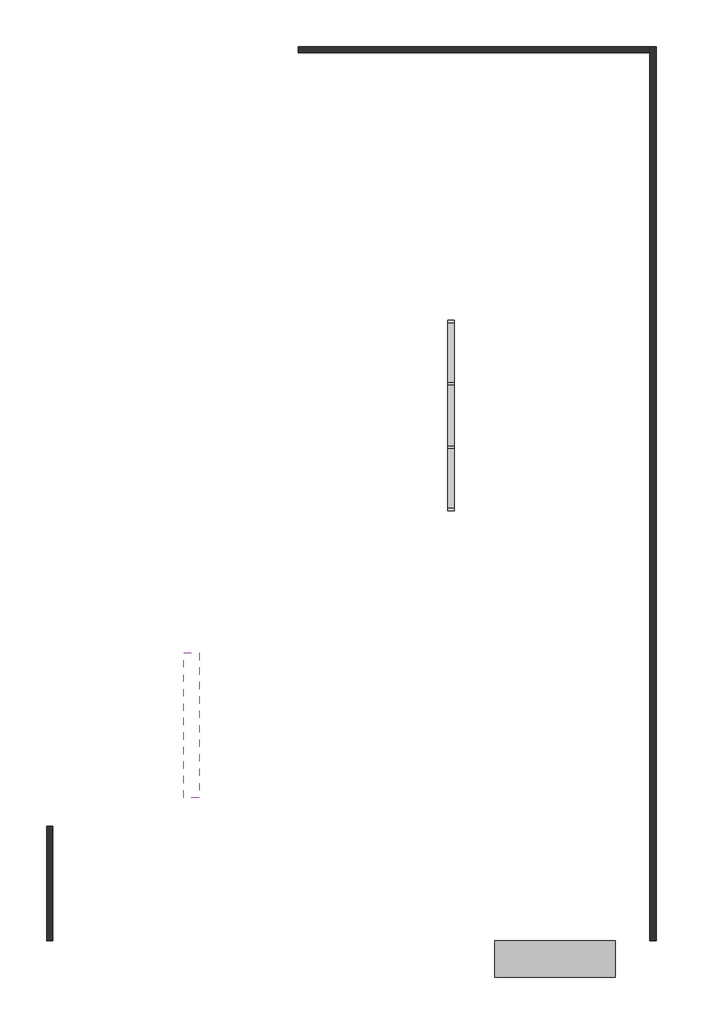
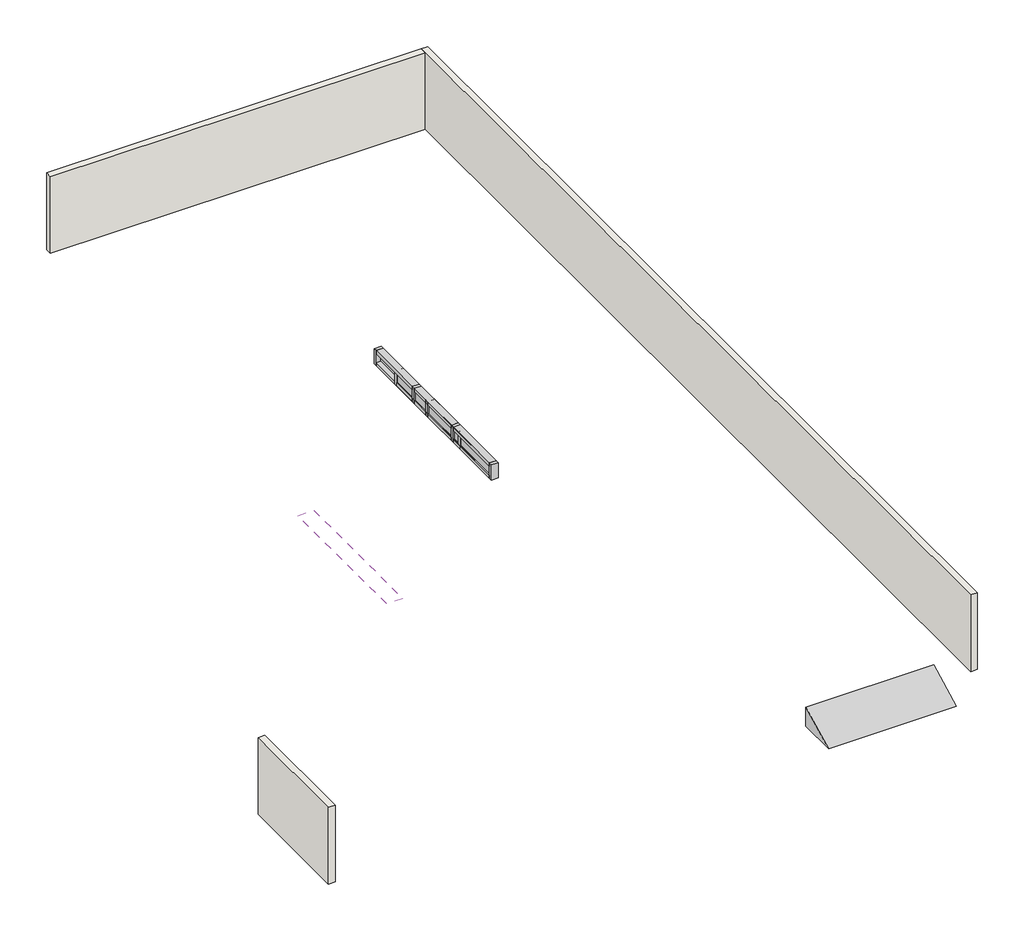
# One storey: 20 members, 6 plates, 3 walls, 1 covering, 1 proxy.
"""IFC4 building model written with IfcOpenShell, lengths in millimetres."""

from ifc_helpers import new_model, si_unit, frame, origin, place, context, project, spatial, polyline, outline, extrude, faceted_brep, transform, mapped, element, save
from components import generic_models_10_generic_models_10_e617d169, member_5d96a33e, member_91edd790, member_75d1e245, member_3c3dc66a, member_3b6b664d, member_f2556e69, system_panel_glazed_cafbbc3c, system_panel_glazed_d1fc495d, system_panel_glazed_eb071a3d, system_panel_glazed_471f9198

model = new_model("IFC4")

# Units and contexts
model_context = context("Model", 3, world=origin())
ifc_project = project(units=[si_unit("LENGTHUNIT", "METRE", prefix="MILLI")], contexts=[model_context])

# Site, building, storey
site = spatial("IfcSite", under=ifc_project)
building = spatial("IfcBuilding", under=site)
storey = spatial("IfcBuildingStorey", under=building, Elevation=0.0)

# Proxy
placement = place(None, origin())
generic_models_10_generic_models_10_shape = generic_models_10_generic_models_10_e617d169(model_context)
element("IfcBuildingElementProxy", 1, Name="Generic Models 10 : Generic Models 10", ObjectType="Generic Models 10 : Generic Models 10", at=placement, inside=storey, context=model_context, shape_type="MappedRepresentation", body=[
    mapped(generic_models_10_generic_models_10_shape, transform((0.0, 0.0, 0.0), x_axis=(1.0, 0.0, 0.0), y_axis=(0.0, 1.0, 0.0), z_axis=(0.0, 0.0, 1.0))),
])

# Covering
element("IfcCovering", 2, at=placement, inside=storey, context=model_context, shape_type="SweptSolid", body=[
    extrude(outline(polyline([(-4259.325552, -303.3614843), (-4259.325552, -3198.9614843), (-4564.125552, -3198.9614843), (-4564.125552, -303.3614843), (-4259.325552, -303.3614843)])), frame((0.0, 0.0, 2870.2), z_axis=(0.0, 0.0, 1.0), x_axis=(1.0, 0.0, 0.0)), (0.0, 0.0, 1.0), 41.275),
    extrude(outline(polyline([(-3649.725552, -303.3614843), (-3649.725552, -3198.9614843), (-3954.525552, -3198.9614843), (-3954.525552, -303.3614843), (-3649.725552, -303.3614843)])), frame((0.0, 0.0, 2870.2), z_axis=(0.0, 0.0, 1.0), x_axis=(1.0, 0.0, 0.0)), (0.0, 0.0, 1.0), 41.275),
    extrude(outline(polyline([(-3065.525552, -303.3614843), (-3065.525552, -3198.9614843), (-3370.325552, -3198.9614843), (-3370.325552, -303.3614843), (-3065.525552, -303.3614843)])), frame((0.0, 0.0, 2870.2), z_axis=(0.0, 0.0, 1.0), x_axis=(1.0, 0.0, 0.0)), (0.0, 0.0, 1.0), 41.275),
    extrude(outline(polyline([(-2455.925552, -303.3614843), (-2455.925552, -3198.9614843), (-2760.725552, -3198.9614843), (-2760.725552, -303.3614843), (-2455.925552, -303.3614843)])), frame((0.0, 0.0, 2870.2), z_axis=(0.0, 0.0, 1.0), x_axis=(1.0, 0.0, 0.0)), (0.0, 0.0, 1.0), 41.275),
    extrude(outline(polyline([(-1846.325552, -303.3614843), (-1846.325552, -3198.9614843), (-2151.125552, -3198.9614843), (-2151.125552, -303.3614843), (-1846.325552, -303.3614843)])), frame((0.0, 0.0, 2870.2), z_axis=(0.0, 0.0, 1.0), x_axis=(1.0, 0.0, 0.0)), (0.0, 0.0, 1.0), 41.275),
    extrude(outline(polyline([(-1236.725552, -303.3614843), (-1236.725552, -3198.9614843), (-1541.525552, -3198.9614843), (-1541.525552, -303.3614843), (-1236.725552, -303.3614843)])), frame((0.0, 0.0, 2870.2), z_axis=(0.0, 0.0, 1.0), x_axis=(1.0, 0.0, 0.0)), (0.0, 0.0, 1.0), 41.275),
])

# Members
member_shape = member_5d96a33e(model_context)
element("IfcMember", 3, ObjectType="Rectangular Mullion : 2.5\" x 5\" rectangular", at=placement, inside=storey, context=model_context, shape_type="MappedRepresentation", body=[
    mapped(member_shape, transform((781.026752, 2602.9133697, 304.8), x_axis=(0.0, 0.0, 1.0), y_axis=(-1.0, 0.0, 0.0), z_axis=(0.0, -1.0, 0.0))),
])
element("IfcMember", 4, ObjectType="Rectangular Mullion : 2.5\" x 5\" rectangular", at=placement, inside=storey, context=model_context, shape_type="MappedRepresentation", body=[
    mapped(member_shape, transform((781.026752, 5111.1633696, 304.8), x_axis=(0.0, 0.0, 1.0), y_axis=(-1.0, 0.0, 0.0), z_axis=(0.0, -1.0, 0.0))),
])
member_2_shape = member_91edd790(model_context)
element("IfcMember", 5, ObjectType="Rectangular Mullion : 2.5\" x 5\" rectangular", at=placement, inside=storey, context=model_context, shape_type="MappedRepresentation", body=[
    mapped(member_2_shape, transform((781.026752, 3841.1633698, 304.8), x_axis=(0.0, 0.0, 1.0), y_axis=(-1.0, 0.0, 0.0), z_axis=(0.0, -1.0, 0.0))),
])
element("IfcMember", 6, ObjectType="Rectangular Mullion : 2.5\" x 5\" rectangular", at=placement, inside=storey, context=model_context, shape_type="MappedRepresentation", body=[
    mapped(member_shape, transform((781.026752, 6285.9133697, 0.0), x_axis=(0.0, 0.0, -1.0), y_axis=(-1.0, 0.0, 0.0), z_axis=(0.0, 1.0, 0.0))),
])
element("IfcMember", 7, ObjectType="Rectangular Mullion : 2.5\" x 5\" rectangular", at=placement, inside=storey, context=model_context, shape_type="MappedRepresentation", body=[
    mapped(member_shape, transform((781.026752, 3777.6633698, 0.0), x_axis=(0.0, 0.0, -1.0), y_axis=(-1.0, 0.0, 0.0), z_axis=(0.0, 1.0, 0.0))),
])
element("IfcMember", 8, ObjectType="Rectangular Mullion : 2.5\" x 5\" rectangular", at=placement, inside=storey, context=model_context, shape_type="MappedRepresentation", body=[
    mapped(member_2_shape, transform((781.026752, 5047.6633696, 0.0), x_axis=(0.0, 0.0, -1.0), y_axis=(-1.0, 0.0, 0.0), z_axis=(0.0, 1.0, 0.0))),
])
member_3_shape = member_75d1e245(model_context)
element("IfcMember", 9, ObjectType="Rectangular Mullion : 2.5\" x 5\" rectangular", at=placement, inside=storey, context=model_context, shape_type="MappedRepresentation", body=[
    mapped(member_3_shape, transform((781.026752, 5079.4133696, 0.0), x_axis=(0.0, -1.0, 0.0), y_axis=(-1.0, 0.0, 0.0), z_axis=(0.0, 0.0, -1.0))),
])
element("IfcMember", 10, ObjectType="Rectangular Mullion : 2.5\" x 5\" rectangular", at=placement, inside=storey, context=model_context, shape_type="MappedRepresentation", body=[
    mapped(member_3_shape, transform((781.026752, 3809.4133698, 0.0), x_axis=(0.0, -1.0, 0.0), y_axis=(-1.0, 0.0, 0.0), z_axis=(0.0, 0.0, -1.0))),
])
element("IfcMember", 11, ObjectType="Rectangular Mullion : 2.5\" x 5\" rectangular", at=placement, inside=storey, context=model_context, shape_type="MappedRepresentation", body=[
    mapped(member_3_shape, transform((781.026752, 3589.2800365, 0.0), x_axis=(0.0, 1.0, 0.0), y_axis=(1.0, 0.0, 0.0), z_axis=(0.0, 0.0, -1.0))),
])
element("IfcMember", 12, ObjectType="Rectangular Mullion : 2.5\" x 5\" rectangular", at=placement, inside=storey, context=model_context, shape_type="MappedRepresentation", body=[
    mapped(member_3_shape, transform((781.026752, 4639.146703, 0.0), x_axis=(0.0, 1.0, 0.0), y_axis=(1.0, 0.0, 0.0), z_axis=(0.0, 0.0, -1.0))),
])
member_4_shape = member_3c3dc66a(model_context)
element("IfcMember", 13, ObjectType="Rectangular Mullion : 2.5\" x 5\" rectangular", at=placement, inside=storey, context=model_context, shape_type="MappedRepresentation", body=[
    mapped(member_4_shape, transform((781.026752, 2539.4133697, 0.0), x_axis=(0.0, -1.0, 0.0), y_axis=(-1.0, 0.0, 0.0), z_axis=(0.0, 0.0, -1.0))),
])
element("IfcMember", 14, ObjectType="Rectangular Mullion : 2.5\" x 5\" rectangular", at=placement, inside=storey, context=model_context, shape_type="MappedRepresentation", body=[
    mapped(member_4_shape, transform((781.026752, 5689.0133697, 0.0), x_axis=(0.0, 1.0, 0.0), y_axis=(1.0, 0.0, 0.0), z_axis=(0.0, 0.0, -1.0))),
])
element("IfcMember", 15, ObjectType="Rectangular Mullion : 2.5\" x 5\" rectangular", at=placement, inside=storey, context=model_context, shape_type="MappedRepresentation", body=[
    mapped(member_4_shape, transform((781.026752, 6349.4133697, 304.8), x_axis=(0.0, 1.0, 0.0), y_axis=(-1.0, 0.0, 0.0), z_axis=(0.0, 0.0, 1.0))),
])
element("IfcMember", 16, ObjectType="Rectangular Mullion : 2.5\" x 5\" rectangular", at=placement, inside=storey, context=model_context, shape_type="MappedRepresentation", body=[
    mapped(member_4_shape, transform((781.026752, 2539.4133697, 304.8), x_axis=(0.0, -1.0, 0.0), y_axis=(1.0, 0.0, 0.0), z_axis=(0.0, 0.0, 1.0))),
])
member_5_shape = member_3b6b664d(model_context)
element("IfcMember", 17, ObjectType="Rectangular Mullion : 2.5\" x 5\" rectangular", at=placement, inside=storey, context=model_context, shape_type="MappedRepresentation", body=[
    mapped(member_5_shape, transform((781.026752, 5625.5133697, 304.8), x_axis=(0.0, 0.0, 1.0), y_axis=(1.0, 0.0, 0.0), z_axis=(0.0, 1.0, 0.0))),
])
element("IfcMember", 18, ObjectType="Rectangular Mullion : 2.5\" x 5\" rectangular", at=placement, inside=storey, context=model_context, shape_type="MappedRepresentation", body=[
    mapped(member_5_shape, transform((781.026752, 3557.5300365, 304.8), x_axis=(0.0, 0.0, 1.0), y_axis=(1.0, 0.0, 0.0), z_axis=(0.0, 1.0, 0.0))),
])
member_6_shape = member_f2556e69(model_context)
element("IfcMember", 19, ObjectType="Rectangular Mullion : 2.5\" x 5\" rectangular", at=placement, inside=storey, context=model_context, shape_type="MappedRepresentation", body=[
    mapped(member_6_shape, transform((781.026752, 4607.396703, 304.8), x_axis=(0.0, 0.0, 1.0), y_axis=(1.0, 0.0, 0.0), z_axis=(0.0, 1.0, 0.0))),
])
element("IfcMember", 20, ObjectType="Rectangular Mullion : 2.5\" x 5\" rectangular", at=placement, inside=storey, context=model_context, shape_type="MappedRepresentation", body=[
    mapped(member_5_shape, transform((781.026752, 2602.9133697, 0.0), x_axis=(0.0, 0.0, -1.0), y_axis=(1.0, 0.0, 0.0), z_axis=(0.0, -1.0, 0.0))),
])
element("IfcMember", 21, ObjectType="Rectangular Mullion : 2.5\" x 5\" rectangular", at=placement, inside=storey, context=model_context, shape_type="MappedRepresentation", body=[
    mapped(member_5_shape, transform((781.026752, 4670.896703, 0.0), x_axis=(0.0, 0.0, -1.0), y_axis=(1.0, 0.0, 0.0), z_axis=(0.0, -1.0, 0.0))),
])
element("IfcMember", 22, ObjectType="Rectangular Mullion : 2.5\" x 5\" rectangular", at=placement, inside=storey, context=model_context, shape_type="MappedRepresentation", body=[
    mapped(member_6_shape, transform((781.026752, 3621.0300365, 0.0), x_axis=(0.0, 0.0, -1.0), y_axis=(1.0, 0.0, 0.0), z_axis=(0.0, -1.0, 0.0))),
])

# Plates
system_panel_glazed_shape = system_panel_glazed_cafbbc3c(model_context)
element("IfcPlate", 23, ObjectType="System Panel : Glazed", at=placement, inside=storey, context=model_context, shape_type="MappedRepresentation", body=[
    mapped(system_panel_glazed_shape, transform((781.026752, 5698.5383697, 63.5), x_axis=(0.0, -1.0, 0.0), y_axis=(1.0, 0.0, 0.0), z_axis=(0.0, 0.0, 1.0))),
])
element("IfcPlate", 24, ObjectType="System Panel : Glazed", at=placement, inside=storey, context=model_context, shape_type="MappedRepresentation", body=[
    mapped(system_panel_glazed_shape, transform((781.026752, 3190.2883698, 63.5), x_axis=(0.0, -1.0, 0.0), y_axis=(1.0, 0.0, 0.0), z_axis=(0.0, 0.0, 1.0))),
])
system_panel_glazed_2_shape = system_panel_glazed_d1fc495d(model_context)
element("IfcPlate", 25, ObjectType="System Panel : Glazed", at=placement, inside=storey, context=model_context, shape_type="MappedRepresentation", body=[
    mapped(system_panel_glazed_2_shape, transform((781.026752, 4444.4133697, 63.5), x_axis=(0.0, -1.0, 0.0), y_axis=(1.0, 0.0, 0.0), z_axis=(0.0, 0.0, 1.0))),
])
system_panel_glazed_3_shape = system_panel_glazed_eb071a3d(model_context)
element("IfcPlate", 26, ObjectType="System Panel : Glazed", at=placement, inside=storey, context=model_context, shape_type="MappedRepresentation", body=[
    mapped(system_panel_glazed_3_shape, transform((781.026752, 3080.2217031, 63.5), x_axis=(0.0, 1.0, 0.0), y_axis=(-1.0, 0.0, 0.0), z_axis=(0.0, 0.0, 1.0))),
])
element("IfcPlate", 27, ObjectType="System Panel : Glazed", at=placement, inside=storey, context=model_context, shape_type="MappedRepresentation", body=[
    mapped(system_panel_glazed_3_shape, transform((781.026752, 5148.2050364, 63.5), x_axis=(0.0, 1.0, 0.0), y_axis=(-1.0, 0.0, 0.0), z_axis=(0.0, 0.0, 1.0))),
])
system_panel_glazed_4_shape = system_panel_glazed_471f9198(model_context)
element("IfcPlate", 28, ObjectType="System Panel : Glazed", at=placement, inside=storey, context=model_context, shape_type="MappedRepresentation", body=[
    mapped(system_panel_glazed_4_shape, transform((781.026752, 4114.2133697, 63.5), x_axis=(0.0, 1.0, 0.0), y_axis=(-1.0, 0.0, 0.0), z_axis=(0.0, 0.0, 1.0))),
])

# Walls
element("IfcWall", 29, ObjectType="INNER WALL 5\"", at=placement, inside=storey, context=model_context, shape_type="Brep", body=[
    faceted_brep([(-7308.873248, -3772.4866303, 0.0), (-7308.873248, -6058.4866303, 0.0), (-7308.873248, -6058.4866303, 1524.0), (-7308.873248, -3772.4866303, 1524.0), (-7308.873248, -3772.4866303, 304.8), (-7181.873248, -3772.4866303, 0.0), (-7181.873248, -3772.4866303, 1524.0), (-7181.873248, -6058.4866303, 1524.0), (-7181.873248, -6058.4866303, 1516.6903378), (-7181.873248, -6058.4866303, 0.0), (-7181.873248, -5931.4866303, 0.0)], [[[0, 1, 2, 3, 4]], [[5, 6, 7, 8, 9, 10]], [[1, 0, 5, 10, 9]], [[3, 2, 7, 6]], [[0, 4, 3, 6, 5]], [[2, 1, 9, 8, 7]]]),
])
element("IfcWall", 30, ObjectType="INNER WALL 5\"", at=placement, inside=storey, context=model_context, shape_type="Brep", body=[
    faceted_brep([(4883.126752, -6058.4866303, 0.0), (4883.126752, 11823.1133697, 0.0), (4883.126752, 11823.1133697, 1524.0), (4883.126752, -6058.4866303, 1524.0), (4756.126752, -6058.4866303, 0.0), (4756.126752, -6058.4866303, 1524.0), (4756.126752, 11696.1133697, 1524.0), (4756.126752, 11823.1133697, 1524.0), (4756.126752, 11823.1133697, 0.0), (4756.126752, 11696.1133697, 0.0), (4756.126752, -5931.4866303, 0.0)], [[[0, 1, 2, 3]], [[4, 5, 6, 7, 8, 9, 10]], [[1, 0, 4, 10, 9, 8]], [[3, 2, 7, 6, 5]], [[2, 1, 8, 7]], [[0, 3, 5, 4]]]),
])
element("IfcWall", 31, ObjectType="INNER WALL 5\"", at=placement, inside=storey, context=model_context, shape_type="Brep", body=[
    faceted_brep([(4756.126752, 11823.1133697, 0.0), (-2279.673248, 11823.1133697, 0.0), (-2279.673248, 11823.1133697, 304.8), (-2279.673248, 11823.1133697, 1524.0), (4756.126752, 11823.1133697, 1524.0), (4756.126752, 11696.1133697, 0.0), (4756.126752, 11696.1133697, 1524.0), (-2279.673248, 11696.1133697, 1524.0), (-2279.673248, 11696.1133697, 0.0)], [[[0, 1, 2, 3, 4]], [[5, 6, 7, 8]], [[1, 0, 5, 8]], [[4, 3, 7, 6]], [[0, 4, 6, 5]], [[3, 2, 1, 8, 7]]]),
])

save(model, "model.ifc")

# Revit data of these elements
# Type
#   Assembly Code = "C3030220"
#   built-in parameter 1002203 = 1 (stored number, unit not read)
#   built-in parameter 1002202 = 1 (stored number, unit not read)
# Type "Rectangular Mullion : 2.5\" x 5\" rectangular"
#   built-in parameter 1007304 = 0.416667 (stored number, unit not read)
#   built-in parameter 1007301 = 0.104167 (stored number, unit not read)
#   built-in parameter 1007300 = 0.104167 (stored number, unit not read)
# Type "System Panel : Glazed"
#   Construction Type Id = "GSP4R"
#   Analytic Construction = "1/8 in Pilkington single glazing"
#   Visual Light Transmittance = 0.9
#   Solar Heat Gain Coefficient = 0.86
#   Heat Transfer Coefficient (U) = 1.18115 BTU/(h·ft²·°F)
#   Define Thermal Properties by = 1
# Type "INNER WALL 5\""
#   Assembly Code = "B2010"
#   Layers, outside or top first: 0' - 5" "IVORY WHITE COLOUR" (function 1)
# Element 1 (IfcBuildingElementProxy, "Generic Models 10 : Generic Models 10")
#   Phase Created = New Construction
#   Materials on its faces: "Concrete, Cast-in-Place gray"
# Element 2 (IfcCovering)
#   Height Offset From Level = 9' - 5"
#   Phase Created = New Construction
# Elements 3, 4, 5, 6, 7, 8, 9, 10, 11, 12, 13, 14, 15, 16, 17, 18, 19, 20, 21, 22 (IfcMember, "Rectangular Mullion : 2.5\" x 5\" rectangular")
#   Phase Created = New Construction
#   Materials on its faces: "Aluminum"
# Elements 23, 24, 25, 26, 27, 28 (IfcPlate, "System Panel : Glazed")
#   Phase Created = New Construction
#   Materials on its faces: "Glass"
# Elements 29, 30, 31 (IfcWall, "INNER WALL 5\"")
#   Top Offset = 0' - 0"
#   Base Offset = 0' - 0"
#   Unconnected Height = 5' - 0"
#   wall height = 5' - 0"
#   Phase Created = New Construction
#   Materials on its faces: "IVORY WHITE COLOUR"
# Materials
#   "IVORY WHITE COLOUR": class "Generic", colour RGB 120 120 120, transparency 0, Cost = 0
#   "Concrete, Cast-in-Place gray": class "Concrete", colour RGB 192 192 192, transparency 0, Description = "Cast-in-place concrete", Cost = 0
#   "Aluminum": class "Metal", colour RGB 247 247 247, transparency 0, Description = "Aluminum 6061", Cost = 0
#   "Glass": class "Glass", colour RGB 0 128 192, transparency 0.75, Description = "Soda Lime Glass", Cost = 0
